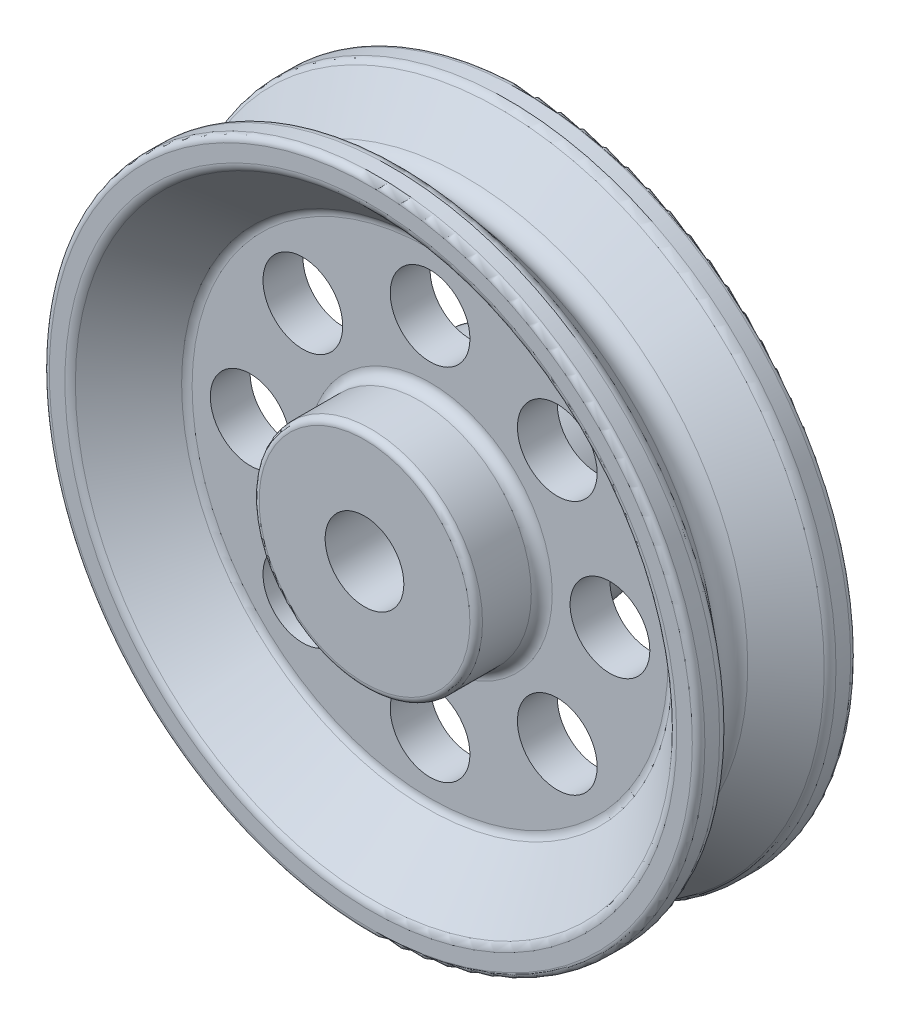
ISO-10303-21;
HEADER;
FILE_DESCRIPTION(('STEP AP214'),'2;1');
FILE_NAME('part.step','',(''),(''),'','','');
FILE_SCHEMA(('AUTOMOTIVE_DESIGN { 1 0 10303 214 1 1 1 1 }'));
ENDSEC;
DATA;
#1=APPLICATION_CONTEXT('core data for automotive mechanical design processes');
#2=APPLICATION_PROTOCOL_DEFINITION('international standard','automotive_design',2000,#1);
#3=PRODUCT_CONTEXT('',#1,'mechanical');
#4=PRODUCT('Part','Part','',(#3));
#5=PRODUCT_RELATED_PRODUCT_CATEGORY('part','',(#4));
#6=PRODUCT_DEFINITION_FORMATION('','',#4);
#7=PRODUCT_DEFINITION_CONTEXT('part definition',#1,'design');
#8=PRODUCT_DEFINITION('design','',#6,#7);
#9=PRODUCT_DEFINITION_SHAPE('','',#8);
#10=(LENGTH_UNIT() NAMED_UNIT(*) SI_UNIT(.MILLI.,.METRE.));
#11=(NAMED_UNIT(*) PLANE_ANGLE_UNIT() SI_UNIT($,.RADIAN.));
#12=(NAMED_UNIT(*) SI_UNIT($,.STERADIAN.) SOLID_ANGLE_UNIT());
#13=UNCERTAINTY_MEASURE_WITH_UNIT(LENGTH_MEASURE(1.E-05),#10,'distance_accuracy_value','');
#14=(GEOMETRIC_REPRESENTATION_CONTEXT(3) GLOBAL_UNCERTAINTY_ASSIGNED_CONTEXT((#13)) GLOBAL_UNIT_ASSIGNED_CONTEXT((#10,
#11,#12)) REPRESENTATION_CONTEXT('',''));
#15=CARTESIAN_POINT('',(0.,0.,0.));
#16=DIRECTION('',(0.,0.,1.));
#17=DIRECTION('',(1.,0.,0.));
#18=AXIS2_PLACEMENT_3D('',#15,#16,#17);
#19=CARTESIAN_POINT('',(0.,1.005,-0.815));
#20=DIRECTION('',(0.,0.,1.));
#21=DIRECTION('',(1.,0.,0.));
#22=AXIS2_PLACEMENT_3D('',#19,#20,#21);
#23=PLANE('',#22);
#24=CARTESIAN_POINT('',(0.,0.,-0.815));
#25=DIRECTION('',(0.,0.,1.));
#26=DIRECTION('',(1.,0.,0.));
#27=AXIS2_PLACEMENT_3D('',#24,#25,#26);
#28=CIRCLE('',#27,1.005);
#29=CARTESIAN_POINT('',(1.005,0.,-0.815));
#30=VERTEX_POINT('',#29);
#31=EDGE_CURVE('E79',#30,#30,#28,.T.);
#32=ORIENTED_EDGE('',*,*,#31,.F.);
#33=EDGE_LOOP('',(#32));
#34=FACE_BOUND('',#33,.T.);
#35=CARTESIAN_POINT('',(0.,0.,-0.815));
#36=DIRECTION('',(0.,0.,1.));
#37=DIRECTION('',(1.,0.,0.));
#38=AXIS2_PLACEMENT_3D('',#35,#36,#37);
#39=CIRCLE('',#38,0.375);
#40=CARTESIAN_POINT('',(0.375,0.,-0.815));
#41=VERTEX_POINT('',#40);
#42=EDGE_CURVE('E10',#41,#41,#39,.T.);
#43=ORIENTED_EDGE('',*,*,#42,.T.);
#44=EDGE_LOOP('',(#43));
#45=FACE_BOUND('',#44,.T.);
#46=ADVANCED_FACE('F40',(#34,#45),#23,.F.);
#47=CARTESIAN_POINT('',(0.,0.,29.1959860355186));
#48=DIRECTION('',(0.,0.,1.));
#49=DIRECTION('',(1.,0.,0.));
#50=AXIS2_PLACEMENT_3D('',#47,#48,#49);
#51=CYLINDRICAL_SURFACE('',#50,0.375);
#52=ORIENTED_EDGE('',*,*,#42,.F.);
#53=EDGE_LOOP('',(#52));
#54=FACE_BOUND('',#53,.T.);
#55=CARTESIAN_POINT('',(0.,0.,0.815));
#56=DIRECTION('',(0.,0.,1.));
#57=DIRECTION('',(1.,0.,0.));
#58=AXIS2_PLACEMENT_3D('',#55,#56,#57);
#59=CIRCLE('',#58,0.375);
#60=CARTESIAN_POINT('',(0.375,0.,0.815));
#61=VERTEX_POINT('',#60);
#62=EDGE_CURVE('E42',#61,#61,#59,.T.);
#63=ORIENTED_EDGE('',*,*,#62,.T.);
#64=EDGE_LOOP('',(#63));
#65=FACE_BOUND('',#64,.T.);
#66=ADVANCED_FACE('F318',(#54,#65),#51,.F.);
#67=CARTESIAN_POINT('',(0.,0.375,0.815));
#68=DIRECTION('',(0.,0.,-1.));
#69=DIRECTION('',(-1.,0.,0.));
#70=AXIS2_PLACEMENT_3D('',#67,#68,#69);
#71=PLANE('',#70);
#72=ORIENTED_EDGE('',*,*,#62,.F.);
#73=EDGE_LOOP('',(#72));
#74=FACE_BOUND('',#73,.T.);
#75=CARTESIAN_POINT('',(0.,0.,0.815));
#76=DIRECTION('',(0.,0.,1.));
#77=DIRECTION('',(1.,0.,0.));
#78=AXIS2_PLACEMENT_3D('',#75,#76,#77);
#79=CIRCLE('',#78,1.005);
#80=CARTESIAN_POINT('',(1.005,0.,0.815));
#81=VERTEX_POINT('',#80);
#82=EDGE_CURVE('E47',#81,#81,#79,.T.);
#83=ORIENTED_EDGE('',*,*,#82,.T.);
#84=EDGE_LOOP('',(#83));
#85=FACE_BOUND('',#84,.T.);
#86=ADVANCED_FACE('F159',(#74,#85),#71,.F.);
#87=CARTESIAN_POINT('',(0.,0.,0.755));
#88=DIRECTION('',(0.,0.,1.));
#89=DIRECTION('',(1.,0.,0.));
#90=AXIS2_PLACEMENT_3D('',#87,#88,#89);
#91=TOROIDAL_SURFACE('',#90,1.005,0.0599999999999999);
#92=ORIENTED_EDGE('',*,*,#82,.F.);
#93=EDGE_LOOP('',(#92));
#94=FACE_BOUND('',#93,.T.);
#95=CARTESIAN_POINT('',(0.,0.,0.754999999999999));
#96=DIRECTION('',(0.,0.,1.));
#97=DIRECTION('',(1.,0.,0.));
#98=AXIS2_PLACEMENT_3D('',#95,#96,#97);
#99=CIRCLE('',#98,1.065);
#100=CARTESIAN_POINT('',(1.065,0.,0.754999999999999));
#101=VERTEX_POINT('',#100);
#102=EDGE_CURVE('E154',#101,#101,#99,.T.);
#103=ORIENTED_EDGE('',*,*,#102,.T.);
#104=EDGE_LOOP('',(#103));
#105=FACE_BOUND('',#104,.T.);
#106=ADVANCED_FACE('F165',(#94,#105),#91,.T.);
#107=CARTESIAN_POINT('',(0.,0.,29.1959860355186));
#108=DIRECTION('',(0.,0.,1.));
#109=DIRECTION('',(1.,0.,0.));
#110=AXIS2_PLACEMENT_3D('',#107,#108,#109);
#111=CYLINDRICAL_SURFACE('',#110,1.065);
#112=ORIENTED_EDGE('',*,*,#102,.F.);
#113=EDGE_LOOP('',(#112));
#114=FACE_BOUND('',#113,.T.);
#115=CARTESIAN_POINT('',(0.,0.,0.290000000000002));
#116=DIRECTION('',(0.,0.,1.));
#117=DIRECTION('',(1.,0.,0.));
#118=AXIS2_PLACEMENT_3D('',#115,#116,#117);
#119=CIRCLE('',#118,1.065);
#120=CARTESIAN_POINT('',(1.065,0.,0.290000000000002));
#121=VERTEX_POINT('',#120);
#122=EDGE_CURVE('E155',#121,#121,#119,.T.);
#123=ORIENTED_EDGE('',*,*,#122,.T.);
#124=EDGE_LOOP('',(#123));
#125=FACE_BOUND('',#124,.T.);
#126=ADVANCED_FACE('F164',(#114,#125),#111,.T.);
#127=CARTESIAN_POINT('',(0.,0.,0.29));
#128=DIRECTION('',(0.,0.,1.));
#129=DIRECTION('',(1.,0.,0.));
#130=AXIS2_PLACEMENT_3D('',#127,#128,#129);
#131=TOROIDAL_SURFACE('',#130,1.165,0.1);
#132=ORIENTED_EDGE('',*,*,#122,.F.);
#133=EDGE_LOOP('',(#132));
#134=FACE_BOUND('',#133,.T.);
#135=CARTESIAN_POINT('',(0.,0.,0.189999999999999));
#136=DIRECTION('',(0.,0.,1.));
#137=DIRECTION('',(1.,0.,0.));
#138=AXIS2_PLACEMENT_3D('',#135,#136,#137);
#139=CIRCLE('',#138,1.165);
#140=CARTESIAN_POINT('',(1.165,0.,0.189999999999999));
#141=VERTEX_POINT('',#140);
#142=EDGE_CURVE('E149',#141,#141,#139,.T.);
#143=ORIENTED_EDGE('',*,*,#142,.T.);
#144=EDGE_LOOP('',(#143));
#145=FACE_BOUND('',#144,.T.);
#146=ADVANCED_FACE('F174',(#134,#145),#131,.F.);
#147=CARTESIAN_POINT('',(0.,1.165,0.19));
#148=DIRECTION('',(0.,0.,-1.));
#149=DIRECTION('',(-1.,0.,0.));
#150=AXIS2_PLACEMENT_3D('',#147,#148,#149);
#151=PLANE('',#150);
#152=CARTESIAN_POINT('',(1.21268812973493,1.21268812973493,0.19));
#153=DIRECTION('',(0.,0.,1.));
#154=DIRECTION('',(1.,0.,0.));
#155=AXIS2_PLACEMENT_3D('',#152,#153,#154);
#156=CIRCLE('',#155,0.38);
#157=CARTESIAN_POINT('',(1.59268812973493,1.21268812973493,0.19));
#158=VERTEX_POINT('',#157);
#159=EDGE_CURVE('E533',#158,#158,#156,.T.);
#160=ORIENTED_EDGE('',*,*,#159,.F.);
#161=EDGE_LOOP('',(#160));
#162=FACE_BOUND('',#161,.T.);
#163=CARTESIAN_POINT('',(1.715,0.,0.19));
#164=DIRECTION('',(0.,0.,1.));
#165=DIRECTION('',(1.,0.,0.));
#166=AXIS2_PLACEMENT_3D('',#163,#164,#165);
#167=CIRCLE('',#166,0.38);
#168=CARTESIAN_POINT('',(2.095,0.,0.19));
#169=VERTEX_POINT('',#168);
#170=EDGE_CURVE('E535',#169,#169,#167,.T.);
#171=ORIENTED_EDGE('',*,*,#170,.F.);
#172=EDGE_LOOP('',(#171));
#173=FACE_BOUND('',#172,.T.);
#174=CARTESIAN_POINT('',(1.21268812973493,-1.21268812973493,0.19));
#175=DIRECTION('',(0.,0.,1.));
#176=DIRECTION('',(1.,0.,0.));
#177=AXIS2_PLACEMENT_3D('',#174,#175,#176);
#178=CIRCLE('',#177,0.38);
#179=CARTESIAN_POINT('',(1.59268812973493,-1.21268812973493,0.19));
#180=VERTEX_POINT('',#179);
#181=EDGE_CURVE('E534',#180,#180,#178,.T.);
#182=ORIENTED_EDGE('',*,*,#181,.F.);
#183=EDGE_LOOP('',(#182));
#184=FACE_BOUND('',#183,.T.);
#185=CARTESIAN_POINT('',(0.,-1.715,0.19));
#186=DIRECTION('',(0.,0.,1.));
#187=DIRECTION('',(1.,0.,0.));
#188=AXIS2_PLACEMENT_3D('',#185,#186,#187);
#189=CIRCLE('',#188,0.38);
#190=CARTESIAN_POINT('',(0.38,-1.715,0.19));
#191=VERTEX_POINT('',#190);
#192=EDGE_CURVE('E537',#191,#191,#189,.T.);
#193=ORIENTED_EDGE('',*,*,#192,.F.);
#194=EDGE_LOOP('',(#193));
#195=FACE_BOUND('',#194,.T.);
#196=CARTESIAN_POINT('',(-1.21268812973493,-1.21268812973493,0.19));
#197=DIRECTION('',(0.,0.,1.));
#198=DIRECTION('',(1.,0.,0.));
#199=AXIS2_PLACEMENT_3D('',#196,#197,#198);
#200=CIRCLE('',#199,0.38);
#201=CARTESIAN_POINT('',(-0.832688129734929,-1.21268812973493,0.19));
#202=VERTEX_POINT('',#201);
#203=EDGE_CURVE('E545',#202,#202,#200,.T.);
#204=ORIENTED_EDGE('',*,*,#203,.F.);
#205=EDGE_LOOP('',(#204));
#206=FACE_BOUND('',#205,.T.);
#207=CARTESIAN_POINT('',(-1.715,0.,0.19));
#208=DIRECTION('',(0.,0.,1.));
#209=DIRECTION('',(1.,0.,0.));
#210=AXIS2_PLACEMENT_3D('',#207,#208,#209);
#211=CIRCLE('',#210,0.38);
#212=CARTESIAN_POINT('',(-1.335,0.,0.19));
#213=VERTEX_POINT('',#212);
#214=EDGE_CURVE('E544',#213,#213,#211,.T.);
#215=ORIENTED_EDGE('',*,*,#214,.F.);
#216=EDGE_LOOP('',(#215));
#217=FACE_BOUND('',#216,.T.);
#218=CARTESIAN_POINT('',(-1.21268812973493,1.21268812973493,0.19));
#219=DIRECTION('',(0.,0.,1.));
#220=DIRECTION('',(1.,0.,0.));
#221=AXIS2_PLACEMENT_3D('',#218,#219,#220);
#222=CIRCLE('',#221,0.38);
#223=CARTESIAN_POINT('',(-0.832688129734929,1.21268812973493,0.19));
#224=VERTEX_POINT('',#223);
#225=EDGE_CURVE('E547',#224,#224,#222,.T.);
#226=ORIENTED_EDGE('',*,*,#225,.F.);
#227=EDGE_LOOP('',(#226));
#228=FACE_BOUND('',#227,.T.);
#229=CARTESIAN_POINT('',(0.,1.715,0.19));
#230=DIRECTION('',(0.,0.,1.));
#231=DIRECTION('',(1.,0.,0.));
#232=AXIS2_PLACEMENT_3D('',#229,#230,#231);
#233=CIRCLE('',#232,0.38);
#234=CARTESIAN_POINT('',(0.38,1.715,0.19));
#235=VERTEX_POINT('',#234);
#236=EDGE_CURVE('E60',#235,#235,#233,.T.);
#237=ORIENTED_EDGE('',*,*,#236,.F.);
#238=EDGE_LOOP('',(#237));
#239=FACE_BOUND('',#238,.T.);
#240=ORIENTED_EDGE('',*,*,#142,.F.);
#241=EDGE_LOOP('',(#240));
#242=FACE_BOUND('',#241,.T.);
#243=CARTESIAN_POINT('',(0.,0.,0.189999999999999));
#244=DIRECTION('',(0.,0.,1.));
#245=DIRECTION('',(1.,0.,0.));
#246=AXIS2_PLACEMENT_3D('',#243,#244,#245);
#247=CIRCLE('',#246,2.26857864376269);
#248=CARTESIAN_POINT('',(2.26857864376269,0.,0.189999999999999));
#249=VERTEX_POINT('',#248);
#250=EDGE_CURVE('E148',#249,#249,#247,.T.);
#251=ORIENTED_EDGE('',*,*,#250,.T.);
#252=EDGE_LOOP('',(#251));
#253=FACE_BOUND('',#252,.T.);
#254=ADVANCED_FACE('F179',(#162,#173,#184,#195,#206,#217,#228,#239,#242,#253),#151,.F.);
#255=CARTESIAN_POINT('',(0.,0.,0.29));
#256=DIRECTION('',(0.,0.,1.));
#257=DIRECTION('',(1.,0.,0.));
#258=AXIS2_PLACEMENT_3D('',#255,#256,#257);
#259=TOROIDAL_SURFACE('',#258,2.26857864376269,0.0999999999999999);
#260=ORIENTED_EDGE('',*,*,#250,.F.);
#261=EDGE_LOOP('',(#260));
#262=FACE_BOUND('',#261,.T.);
#263=CARTESIAN_POINT('',(0.,0.,0.219289321881345));
#264=DIRECTION('',(0.,0.,1.));
#265=DIRECTION('',(1.,0.,0.));
#266=AXIS2_PLACEMENT_3D('',#263,#264,#265);
#267=CIRCLE('',#266,2.33928932188135);
#268=CARTESIAN_POINT('',(2.33928932188135,0.,0.219289321881345));
#269=VERTEX_POINT('',#268);
#270=EDGE_CURVE('E141',#269,#269,#267,.T.);
#271=ORIENTED_EDGE('',*,*,#270,.T.);
#272=EDGE_LOOP('',(#271));
#273=FACE_BOUND('',#272,.T.);
#274=ADVANCED_FACE('F181',(#262,#273),#259,.F.);
#275=CARTESIAN_POINT('',(0.,0.,0.725710678118652));
#276=DIRECTION('',(0.,0.,1.));
#277=DIRECTION('',(1.,0.,0.));
#278=AXIS2_PLACEMENT_3D('',#275,#276,#277);
#279=CONICAL_SURFACE('',#278,2.84571067811865,0.785398163397448);
#280=ORIENTED_EDGE('',*,*,#270,.F.);
#281=EDGE_LOOP('',(#280));
#282=FACE_BOUND('',#281,.T.);
#283=CARTESIAN_POINT('',(0.,0.,0.725710678118652));
#284=DIRECTION('',(0.,0.,1.));
#285=DIRECTION('',(1.,0.,0.));
#286=AXIS2_PLACEMENT_3D('',#283,#284,#285);
#287=CIRCLE('',#286,2.84571067811865);
#288=CARTESIAN_POINT('',(2.84571067811865,0.,0.725710678118652));
#289=VERTEX_POINT('',#288);
#290=EDGE_CURVE('E138',#289,#289,#287,.T.);
#291=ORIENTED_EDGE('',*,*,#290,.T.);
#292=EDGE_LOOP('',(#291));
#293=FACE_BOUND('',#292,.T.);
#294=ADVANCED_FACE('F187',(#282,#293),#279,.F.);
#295=CARTESIAN_POINT('',(0.,0.,0.655));
#296=DIRECTION('',(0.,0.,1.));
#297=DIRECTION('',(1.,0.,0.));
#298=AXIS2_PLACEMENT_3D('',#295,#296,#297);
#299=TOROIDAL_SURFACE('',#298,2.91642135623731,0.1);
#300=ORIENTED_EDGE('',*,*,#290,.F.);
#301=EDGE_LOOP('',(#300));
#302=FACE_BOUND('',#301,.T.);
#303=CARTESIAN_POINT('',(0.,0.,0.754999999999999));
#304=DIRECTION('',(0.,0.,1.));
#305=DIRECTION('',(1.,0.,0.));
#306=AXIS2_PLACEMENT_3D('',#303,#304,#305);
#307=CIRCLE('',#306,2.91642135623731);
#308=CARTESIAN_POINT('',(2.91642135623731,0.,0.754999999999999));
#309=VERTEX_POINT('',#308);
#310=EDGE_CURVE('E139',#309,#309,#307,.T.);
#311=ORIENTED_EDGE('',*,*,#310,.T.);
#312=EDGE_LOOP('',(#311));
#313=FACE_BOUND('',#312,.T.);
#314=ADVANCED_FACE('F198',(#302,#313),#299,.T.);
#315=CARTESIAN_POINT('',(0.,2.91642135623731,0.754999999999999));
#316=DIRECTION('',(0.,0.,-1.));
#317=DIRECTION('',(-1.,0.,0.));
#318=AXIS2_PLACEMENT_3D('',#315,#316,#317);
#319=PLANE('',#318);
#320=ORIENTED_EDGE('',*,*,#310,.F.);
#321=EDGE_LOOP('',(#320));
#322=FACE_BOUND('',#321,.T.);
#323=CARTESIAN_POINT('',(0.,0.,0.754999999999999));
#324=DIRECTION('',(0.,0.,1.));
#325=DIRECTION('',(1.,0.,0.));
#326=AXIS2_PLACEMENT_3D('',#323,#324,#325);
#327=CIRCLE('',#326,3.065);
#328=CARTESIAN_POINT('',(3.065,0.,0.754999999999999));
#329=VERTEX_POINT('',#328);
#330=EDGE_CURVE('E133',#329,#329,#327,.T.);
#331=ORIENTED_EDGE('',*,*,#330,.T.);
#332=EDGE_LOOP('',(#331));
#333=FACE_BOUND('',#332,.T.);
#334=ADVANCED_FACE('F205',(#322,#333),#319,.F.);
#335=CARTESIAN_POINT('',(0.,0.,0.694999999999999));
#336=DIRECTION('',(0.,0.,1.));
#337=DIRECTION('',(1.,0.,0.));
#338=AXIS2_PLACEMENT_3D('',#335,#336,#337);
#339=TOROIDAL_SURFACE('',#338,3.065,0.06);
#340=ORIENTED_EDGE('',*,*,#330,.F.);
#341=EDGE_LOOP('',(#340));
#342=FACE_BOUND('',#341,.T.);
#343=CARTESIAN_POINT('',(0.,0.,0.694999999999998));
#344=DIRECTION('',(0.,0.,1.));
#345=DIRECTION('',(1.,0.,0.));
#346=AXIS2_PLACEMENT_3D('',#343,#344,#345);
#347=CIRCLE('',#346,3.125);
#348=CARTESIAN_POINT('',(3.125,0.,0.694999999999998));
#349=VERTEX_POINT('',#348);
#350=EDGE_CURVE('E134',#349,#349,#347,.T.);
#351=ORIENTED_EDGE('',*,*,#350,.T.);
#352=EDGE_LOOP('',(#351));
#353=FACE_BOUND('',#352,.T.);
#354=ADVANCED_FACE('F208',(#342,#353),#339,.T.);
#355=CARTESIAN_POINT('',(0.,0.,29.1959860355186));
#356=DIRECTION('',(0.,0.,1.));
#357=DIRECTION('',(1.,0.,0.));
#358=AXIS2_PLACEMENT_3D('',#355,#356,#357);
#359=CYLINDRICAL_SURFACE('',#358,3.125);
#360=ORIENTED_EDGE('',*,*,#350,.F.);
#361=EDGE_LOOP('',(#360));
#362=FACE_BOUND('',#361,.T.);
#363=CARTESIAN_POINT('',(0.,0.,0.554779036453578));
#364=DIRECTION('',(0.,0.,1.));
#365=DIRECTION('',(1.,0.,0.));
#366=AXIS2_PLACEMENT_3D('',#363,#364,#365);
#367=CIRCLE('',#366,3.125);
#368=CARTESIAN_POINT('',(3.125,0.,0.554779036453578));
#369=VERTEX_POINT('',#368);
#370=EDGE_CURVE('E126',#369,#369,#367,.T.);
#371=ORIENTED_EDGE('',*,*,#370,.T.);
#372=EDGE_LOOP('',(#371));
#373=FACE_BOUND('',#372,.T.);
#374=ADVANCED_FACE('F212',(#362,#373),#359,.T.);
#375=CARTESIAN_POINT('',(0.,0.,0.554779036453579));
#376=DIRECTION('',(0.,0.,1.));
#377=DIRECTION('',(1.,0.,0.));
#378=AXIS2_PLACEMENT_3D('',#375,#376,#377);
#379=TOROIDAL_SURFACE('',#378,3.025,0.0999999999999998);
#380=ORIENTED_EDGE('',*,*,#370,.F.);
#381=EDGE_LOOP('',(#380));
#382=FACE_BOUND('',#381,.T.);
#383=CARTESIAN_POINT('',(0.,0.,0.478174592141681));
#384=DIRECTION('',(0.,0.,1.));
#385=DIRECTION('',(1.,0.,0.));
#386=AXIS2_PLACEMENT_3D('',#383,#384,#385);
#387=CIRCLE('',#386,3.08927876096865);
#388=CARTESIAN_POINT('',(3.08927876096865,0.,0.478174592141681));
#389=VERTEX_POINT('',#388);
#390=EDGE_CURVE('E123',#389,#389,#387,.T.);
#391=ORIENTED_EDGE('',*,*,#390,.T.);
#392=EDGE_LOOP('',(#391));
#393=FACE_BOUND('',#392,.T.);
#394=ADVANCED_FACE('F219',(#382,#393),#379,.T.);
#395=CARTESIAN_POINT('',(0.,0.,0.145548444192605));
#396=DIRECTION('',(0.,0.,1.));
#397=DIRECTION('',(1.,0.,0.));
#398=AXIS2_PLACEMENT_3D('',#395,#396,#397);
#399=CONICAL_SURFACE('',#398,2.69287035415956,0.872664625997176);
#400=ORIENTED_EDGE('',*,*,#390,.F.);
#401=EDGE_LOOP('',(#400));
#402=FACE_BOUND('',#401,.T.);
#403=CARTESIAN_POINT('',(0.,0.,0.145548444192605));
#404=DIRECTION('',(0.,0.,1.));
#405=DIRECTION('',(1.,0.,0.));
#406=AXIS2_PLACEMENT_3D('',#403,#404,#405);
#407=CIRCLE('',#406,2.69287035415956);
#408=CARTESIAN_POINT('',(2.69287035415956,0.,0.145548444192605));
#409=VERTEX_POINT('',#408);
#410=EDGE_CURVE('E124',#409,#409,#407,.T.);
#411=ORIENTED_EDGE('',*,*,#410,.T.);
#412=EDGE_LOOP('',(#411));
#413=FACE_BOUND('',#412,.T.);
#414=ADVANCED_FACE('F229',(#402,#413),#399,.T.);
#415=CARTESIAN_POINT('',(0.,0.,0.));
#416=DIRECTION('',(0.,0.,1.));
#417=DIRECTION('',(1.,0.,0.));
#418=AXIS2_PLACEMENT_3D('',#415,#416,#417);
#419=TOROIDAL_SURFACE('',#418,2.815,0.189999999999999);
#420=ORIENTED_EDGE('',*,*,#410,.F.);
#421=EDGE_LOOP('',(#420));
#422=FACE_BOUND('',#421,.T.);
#423=CARTESIAN_POINT('',(0.,0.,-0.145548444192605));
#424=DIRECTION('',(0.,0.,1.));
#425=DIRECTION('',(1.,0.,0.));
#426=AXIS2_PLACEMENT_3D('',#423,#424,#425);
#427=CIRCLE('',#426,2.69287035415956);
#428=CARTESIAN_POINT('',(2.69287035415956,0.,-0.145548444192605));
#429=VERTEX_POINT('',#428);
#430=EDGE_CURVE('E118',#429,#429,#427,.T.);
#431=ORIENTED_EDGE('',*,*,#430,.T.);
#432=EDGE_LOOP('',(#431));
#433=FACE_BOUND('',#432,.T.);
#434=ADVANCED_FACE('F234',(#422,#433),#419,.F.);
#435=CARTESIAN_POINT('',(0.,0.,-0.478174592141702));
#436=DIRECTION('',(0.,0.,-1.));
#437=DIRECTION('',(-1.,0.,0.));
#438=AXIS2_PLACEMENT_3D('',#435,#436,#437);
#439=CONICAL_SURFACE('',#438,3.08927876096866,0.872664625997154);
#440=ORIENTED_EDGE('',*,*,#430,.F.);
#441=EDGE_LOOP('',(#440));
#442=FACE_BOUND('',#441,.T.);
#443=CARTESIAN_POINT('',(0.,0.,-0.478174592141702));
#444=DIRECTION('',(0.,0.,1.));
#445=DIRECTION('',(1.,0.,0.));
#446=AXIS2_PLACEMENT_3D('',#443,#444,#445);
#447=CIRCLE('',#446,3.08927876096866);
#448=CARTESIAN_POINT('',(3.08927876096866,0.,-0.478174592141702));
#449=VERTEX_POINT('',#448);
#450=EDGE_CURVE('E119',#449,#449,#447,.T.);
#451=ORIENTED_EDGE('',*,*,#450,.T.);
#452=EDGE_LOOP('',(#451));
#453=FACE_BOUND('',#452,.T.);
#454=ADVANCED_FACE('F236',(#442,#453),#439,.T.);
#455=CARTESIAN_POINT('',(0.,0.,-0.554779036453598));
#456=DIRECTION('',(0.,0.,1.));
#457=DIRECTION('',(1.,0.,0.));
#458=AXIS2_PLACEMENT_3D('',#455,#456,#457);
#459=TOROIDAL_SURFACE('',#458,3.025,0.0999999999999998);
#460=ORIENTED_EDGE('',*,*,#450,.F.);
#461=EDGE_LOOP('',(#460));
#462=FACE_BOUND('',#461,.T.);
#463=CARTESIAN_POINT('',(0.,0.,-0.554779036453599));
#464=DIRECTION('',(0.,0.,1.));
#465=DIRECTION('',(1.,0.,0.));
#466=AXIS2_PLACEMENT_3D('',#463,#464,#465);
#467=CIRCLE('',#466,3.125);
#468=CARTESIAN_POINT('',(3.125,0.,-0.554779036453599));
#469=VERTEX_POINT('',#468);
#470=EDGE_CURVE('E114',#469,#469,#467,.T.);
#471=ORIENTED_EDGE('',*,*,#470,.T.);
#472=EDGE_LOOP('',(#471));
#473=FACE_BOUND('',#472,.T.);
#474=ADVANCED_FACE('F243',(#462,#473),#459,.T.);
#475=CARTESIAN_POINT('',(0.,0.,29.1959860355186));
#476=DIRECTION('',(0.,0.,1.));
#477=DIRECTION('',(1.,0.,0.));
#478=AXIS2_PLACEMENT_3D('',#475,#476,#477);
#479=CYLINDRICAL_SURFACE('',#478,3.125);
#480=ORIENTED_EDGE('',*,*,#470,.F.);
#481=EDGE_LOOP('',(#480));
#482=FACE_BOUND('',#481,.T.);
#483=CARTESIAN_POINT('',(0.,0.,-0.695000000000001));
#484=DIRECTION('',(0.,0.,1.));
#485=DIRECTION('',(1.,0.,0.));
#486=AXIS2_PLACEMENT_3D('',#483,#484,#485);
#487=CIRCLE('',#486,3.125);
#488=CARTESIAN_POINT('',(3.125,0.,-0.695000000000001));
#489=VERTEX_POINT('',#488);
#490=EDGE_CURVE('E109',#489,#489,#487,.T.);
#491=ORIENTED_EDGE('',*,*,#490,.T.);
#492=EDGE_LOOP('',(#491));
#493=FACE_BOUND('',#492,.T.);
#494=ADVANCED_FACE('F248',(#482,#493),#479,.T.);
#495=CARTESIAN_POINT('',(0.,0.,-0.695));
#496=DIRECTION('',(0.,0.,1.));
#497=DIRECTION('',(1.,0.,0.));
#498=AXIS2_PLACEMENT_3D('',#495,#496,#497);
#499=TOROIDAL_SURFACE('',#498,3.065,0.06);
#500=ORIENTED_EDGE('',*,*,#490,.F.);
#501=EDGE_LOOP('',(#500));
#502=FACE_BOUND('',#501,.T.);
#503=CARTESIAN_POINT('',(0.,0.,-0.754999999999999));
#504=DIRECTION('',(0.,0.,1.));
#505=DIRECTION('',(1.,0.,0.));
#506=AXIS2_PLACEMENT_3D('',#503,#504,#505);
#507=CIRCLE('',#506,3.065);
#508=CARTESIAN_POINT('',(3.065,0.,-0.754999999999999));
#509=VERTEX_POINT('',#508);
#510=EDGE_CURVE('E110',#509,#509,#507,.T.);
#511=ORIENTED_EDGE('',*,*,#510,.T.);
#512=EDGE_LOOP('',(#511));
#513=FACE_BOUND('',#512,.T.);
#514=ADVANCED_FACE('F258',(#502,#513),#499,.T.);
#515=CARTESIAN_POINT('',(0.,3.065,-0.755));
#516=DIRECTION('',(0.,0.,1.));
#517=DIRECTION('',(1.,0.,0.));
#518=AXIS2_PLACEMENT_3D('',#515,#516,#517);
#519=PLANE('',#518);
#520=ORIENTED_EDGE('',*,*,#510,.F.);
#521=EDGE_LOOP('',(#520));
#522=FACE_BOUND('',#521,.T.);
#523=CARTESIAN_POINT('',(0.,0.,-0.754999999999999));
#524=DIRECTION('',(0.,0.,1.));
#525=DIRECTION('',(1.,0.,0.));
#526=AXIS2_PLACEMENT_3D('',#523,#524,#525);
#527=CIRCLE('',#526,2.91642135623731);
#528=CARTESIAN_POINT('',(2.91642135623731,0.,-0.754999999999999));
#529=VERTEX_POINT('',#528);
#530=EDGE_CURVE('E102',#529,#529,#527,.T.);
#531=ORIENTED_EDGE('',*,*,#530,.T.);
#532=EDGE_LOOP('',(#531));
#533=FACE_BOUND('',#532,.T.);
#534=ADVANCED_FACE('F265',(#522,#533),#519,.F.);
#535=CARTESIAN_POINT('',(0.,0.,-0.655));
#536=DIRECTION('',(0.,0.,1.));
#537=DIRECTION('',(1.,0.,0.));
#538=AXIS2_PLACEMENT_3D('',#535,#536,#537);
#539=TOROIDAL_SURFACE('',#538,2.91642135623731,0.0999999999999999);
#540=ORIENTED_EDGE('',*,*,#530,.F.);
#541=EDGE_LOOP('',(#540));
#542=FACE_BOUND('',#541,.T.);
#543=CARTESIAN_POINT('',(0.,0.,-0.725710678118656));
#544=DIRECTION('',(0.,0.,1.));
#545=DIRECTION('',(1.,0.,0.));
#546=AXIS2_PLACEMENT_3D('',#543,#544,#545);
#547=CIRCLE('',#546,2.84571067811865);
#548=CARTESIAN_POINT('',(2.84571067811865,0.,-0.725710678118656));
#549=VERTEX_POINT('',#548);
#550=EDGE_CURVE('E101',#549,#549,#547,.T.);
#551=ORIENTED_EDGE('',*,*,#550,.T.);
#552=EDGE_LOOP('',(#551));
#553=FACE_BOUND('',#552,.T.);
#554=ADVANCED_FACE('F268',(#542,#553),#539,.T.);
#555=CARTESIAN_POINT('',(0.,0.,-0.219289321881345));
#556=DIRECTION('',(0.,0.,-1.));
#557=DIRECTION('',(-1.,0.,0.));
#558=AXIS2_PLACEMENT_3D('',#555,#556,#557);
#559=CONICAL_SURFACE('',#558,2.33928932188135,0.785398163397446);
#560=ORIENTED_EDGE('',*,*,#550,.F.);
#561=EDGE_LOOP('',(#560));
#562=FACE_BOUND('',#561,.T.);
#563=CARTESIAN_POINT('',(0.,0.,-0.219289321881345));
#564=DIRECTION('',(0.,0.,1.));
#565=DIRECTION('',(1.,0.,0.));
#566=AXIS2_PLACEMENT_3D('',#563,#564,#565);
#567=CIRCLE('',#566,2.33928932188135);
#568=CARTESIAN_POINT('',(2.33928932188135,0.,-0.219289321881345));
#569=VERTEX_POINT('',#568);
#570=EDGE_CURVE('E98',#569,#569,#567,.T.);
#571=ORIENTED_EDGE('',*,*,#570,.T.);
#572=EDGE_LOOP('',(#571));
#573=FACE_BOUND('',#572,.T.);
#574=ADVANCED_FACE('F273',(#562,#573),#559,.F.);
#575=CARTESIAN_POINT('',(0.,0.,-0.29));
#576=DIRECTION('',(0.,0.,1.));
#577=DIRECTION('',(1.,0.,0.));
#578=AXIS2_PLACEMENT_3D('',#575,#576,#577);
#579=TOROIDAL_SURFACE('',#578,2.26857864376269,0.0999999999999999);
#580=ORIENTED_EDGE('',*,*,#570,.F.);
#581=EDGE_LOOP('',(#580));
#582=FACE_BOUND('',#581,.T.);
#583=CARTESIAN_POINT('',(0.,0.,-0.189999999999999));
#584=DIRECTION('',(0.,0.,1.));
#585=DIRECTION('',(1.,0.,0.));
#586=AXIS2_PLACEMENT_3D('',#583,#584,#585);
#587=CIRCLE('',#586,2.26857864376269);
#588=CARTESIAN_POINT('',(2.26857864376269,0.,-0.189999999999999));
#589=VERTEX_POINT('',#588);
#590=EDGE_CURVE('E92',#589,#589,#587,.T.);
#591=ORIENTED_EDGE('',*,*,#590,.T.);
#592=EDGE_LOOP('',(#591));
#593=FACE_BOUND('',#592,.T.);
#594=ADVANCED_FACE('F278',(#582,#593),#579,.F.);
#595=CARTESIAN_POINT('',(0.,2.26857864376269,-0.19));
#596=DIRECTION('',(0.,0.,1.));
#597=DIRECTION('',(1.,0.,0.));
#598=AXIS2_PLACEMENT_3D('',#595,#596,#597);
#599=PLANE('',#598);
#600=CARTESIAN_POINT('',(1.21268812973493,1.21268812973493,-0.19));
#601=DIRECTION('',(0.,0.,1.));
#602=DIRECTION('',(1.,0.,0.));
#603=AXIS2_PLACEMENT_3D('',#600,#601,#602);
#604=CIRCLE('',#603,0.38);
#605=CARTESIAN_POINT('',(1.59268812973493,1.21268812973493,-0.19));
#606=VERTEX_POINT('',#605);
#607=EDGE_CURVE('E37',#606,#606,#604,.T.);
#608=ORIENTED_EDGE('',*,*,#607,.T.);
#609=EDGE_LOOP('',(#608));
#610=FACE_BOUND('',#609,.T.);
#611=CARTESIAN_POINT('',(1.715,0.,-0.19));
#612=DIRECTION('',(0.,0.,1.));
#613=DIRECTION('',(1.,0.,0.));
#614=AXIS2_PLACEMENT_3D('',#611,#612,#613);
#615=CIRCLE('',#614,0.38);
#616=CARTESIAN_POINT('',(2.095,0.,-0.19));
#617=VERTEX_POINT('',#616);
#618=EDGE_CURVE('E72',#617,#617,#615,.T.);
#619=ORIENTED_EDGE('',*,*,#618,.T.);
#620=EDGE_LOOP('',(#619));
#621=FACE_BOUND('',#620,.T.);
#622=CARTESIAN_POINT('',(1.21268812973493,-1.21268812973493,-0.19));
#623=DIRECTION('',(0.,0.,1.));
#624=DIRECTION('',(1.,0.,0.));
#625=AXIS2_PLACEMENT_3D('',#622,#623,#624);
#626=CIRCLE('',#625,0.38);
#627=CARTESIAN_POINT('',(1.59268812973493,-1.21268812973493,-0.19));
#628=VERTEX_POINT('',#627);
#629=EDGE_CURVE('E66',#628,#628,#626,.T.);
#630=ORIENTED_EDGE('',*,*,#629,.T.);
#631=EDGE_LOOP('',(#630));
#632=FACE_BOUND('',#631,.T.);
#633=CARTESIAN_POINT('',(0.,-1.715,-0.19));
#634=DIRECTION('',(0.,0.,1.));
#635=DIRECTION('',(1.,0.,0.));
#636=AXIS2_PLACEMENT_3D('',#633,#634,#635);
#637=CIRCLE('',#636,0.38);
#638=CARTESIAN_POINT('',(0.38,-1.715,-0.19));
#639=VERTEX_POINT('',#638);
#640=EDGE_CURVE('E67',#639,#639,#637,.T.);
#641=ORIENTED_EDGE('',*,*,#640,.T.);
#642=EDGE_LOOP('',(#641));
#643=FACE_BOUND('',#642,.T.);
#644=CARTESIAN_POINT('',(-1.21268812973493,-1.21268812973493,-0.19));
#645=DIRECTION('',(0.,0.,1.));
#646=DIRECTION('',(1.,0.,0.));
#647=AXIS2_PLACEMENT_3D('',#644,#645,#646);
#648=CIRCLE('',#647,0.38);
#649=CARTESIAN_POINT('',(-0.832688129734929,-1.21268812973493,-0.19));
#650=VERTEX_POINT('',#649);
#651=EDGE_CURVE('E65',#650,#650,#648,.T.);
#652=ORIENTED_EDGE('',*,*,#651,.T.);
#653=EDGE_LOOP('',(#652));
#654=FACE_BOUND('',#653,.T.);
#655=CARTESIAN_POINT('',(-1.715,0.,-0.19));
#656=DIRECTION('',(0.,0.,1.));
#657=DIRECTION('',(1.,0.,0.));
#658=AXIS2_PLACEMENT_3D('',#655,#656,#657);
#659=CIRCLE('',#658,0.38);
#660=CARTESIAN_POINT('',(-1.335,0.,-0.19));
#661=VERTEX_POINT('',#660);
#662=EDGE_CURVE('E58',#661,#661,#659,.T.);
#663=ORIENTED_EDGE('',*,*,#662,.T.);
#664=EDGE_LOOP('',(#663));
#665=FACE_BOUND('',#664,.T.);
#666=CARTESIAN_POINT('',(-1.21268812973493,1.21268812973493,-0.19));
#667=DIRECTION('',(0.,0.,1.));
#668=DIRECTION('',(1.,0.,0.));
#669=AXIS2_PLACEMENT_3D('',#666,#667,#668);
#670=CIRCLE('',#669,0.38);
#671=CARTESIAN_POINT('',(-0.832688129734929,1.21268812973493,-0.19));
#672=VERTEX_POINT('',#671);
#673=EDGE_CURVE('E57',#672,#672,#670,.T.);
#674=ORIENTED_EDGE('',*,*,#673,.T.);
#675=EDGE_LOOP('',(#674));
#676=FACE_BOUND('',#675,.T.);
#677=CARTESIAN_POINT('',(0.,1.715,-0.19));
#678=DIRECTION('',(0.,0.,1.));
#679=DIRECTION('',(1.,0.,0.));
#680=AXIS2_PLACEMENT_3D('',#677,#678,#679);
#681=CIRCLE('',#680,0.38);
#682=CARTESIAN_POINT('',(0.38,1.715,-0.19));
#683=VERTEX_POINT('',#682);
#684=EDGE_CURVE('E52',#683,#683,#681,.T.);
#685=ORIENTED_EDGE('',*,*,#684,.T.);
#686=EDGE_LOOP('',(#685));
#687=FACE_BOUND('',#686,.T.);
#688=ORIENTED_EDGE('',*,*,#590,.F.);
#689=EDGE_LOOP('',(#688));
#690=FACE_BOUND('',#689,.T.);
#691=CARTESIAN_POINT('',(0.,0.,-0.189999999999999));
#692=DIRECTION('',(0.,0.,1.));
#693=DIRECTION('',(1.,0.,0.));
#694=AXIS2_PLACEMENT_3D('',#691,#692,#693);
#695=CIRCLE('',#694,1.165);
#696=CARTESIAN_POINT('',(1.165,0.,-0.189999999999999));
#697=VERTEX_POINT('',#696);
#698=EDGE_CURVE('E95',#697,#697,#695,.T.);
#699=ORIENTED_EDGE('',*,*,#698,.T.);
#700=EDGE_LOOP('',(#699));
#701=FACE_BOUND('',#700,.T.);
#702=ADVANCED_FACE('F287',(#610,#621,#632,#643,#654,#665,#676,#687,#690,#701),#599,.F.);
#703=CARTESIAN_POINT('',(0.,0.,-0.29));
#704=DIRECTION('',(0.,0.,1.));
#705=DIRECTION('',(1.,0.,0.));
#706=AXIS2_PLACEMENT_3D('',#703,#704,#705);
#707=TOROIDAL_SURFACE('',#706,1.165,0.1);
#708=ORIENTED_EDGE('',*,*,#698,.F.);
#709=EDGE_LOOP('',(#708));
#710=FACE_BOUND('',#709,.T.);
#711=CARTESIAN_POINT('',(0.,0.,-0.290000000000002));
#712=DIRECTION('',(0.,0.,1.));
#713=DIRECTION('',(1.,0.,0.));
#714=AXIS2_PLACEMENT_3D('',#711,#712,#713);
#715=CIRCLE('',#714,1.065);
#716=CARTESIAN_POINT('',(1.065,0.,-0.290000000000002));
#717=VERTEX_POINT('',#716);
#718=EDGE_CURVE('E83',#717,#717,#715,.T.);
#719=ORIENTED_EDGE('',*,*,#718,.T.);
#720=EDGE_LOOP('',(#719));
#721=FACE_BOUND('',#720,.T.);
#722=ADVANCED_FACE('F295',(#710,#721),#707,.F.);
#723=CARTESIAN_POINT('',(0.,0.,29.1959860355186));
#724=DIRECTION('',(0.,0.,1.));
#725=DIRECTION('',(1.,0.,0.));
#726=AXIS2_PLACEMENT_3D('',#723,#724,#725);
#727=CYLINDRICAL_SURFACE('',#726,1.065);
#728=ORIENTED_EDGE('',*,*,#718,.F.);
#729=EDGE_LOOP('',(#728));
#730=FACE_BOUND('',#729,.T.);
#731=CARTESIAN_POINT('',(0.,0.,-0.754999999999999));
#732=DIRECTION('',(0.,0.,1.));
#733=DIRECTION('',(1.,0.,0.));
#734=AXIS2_PLACEMENT_3D('',#731,#732,#733);
#735=CIRCLE('',#734,1.065);
#736=CARTESIAN_POINT('',(1.065,0.,-0.754999999999999));
#737=VERTEX_POINT('',#736);
#738=EDGE_CURVE('E77',#737,#737,#735,.T.);
#739=ORIENTED_EDGE('',*,*,#738,.T.);
#740=EDGE_LOOP('',(#739));
#741=FACE_BOUND('',#740,.T.);
#742=ADVANCED_FACE('F300',(#730,#741),#727,.T.);
#743=CARTESIAN_POINT('',(0.,0.,-0.755));
#744=DIRECTION('',(0.,0.,1.));
#745=DIRECTION('',(1.,0.,0.));
#746=AXIS2_PLACEMENT_3D('',#743,#744,#745);
#747=TOROIDAL_SURFACE('',#746,1.005,0.0599999999999999);
#748=ORIENTED_EDGE('',*,*,#738,.F.);
#749=EDGE_LOOP('',(#748));
#750=FACE_BOUND('',#749,.T.);
#751=ORIENTED_EDGE('',*,*,#31,.T.);
#752=EDGE_LOOP('',(#751));
#753=FACE_BOUND('',#752,.T.);
#754=ADVANCED_FACE('F301',(#750,#753),#747,.T.);
#755=CARTESIAN_POINT('',(0.,1.715,-0.815));
#756=DIRECTION('',(0.,0.,1.));
#757=DIRECTION('',(1.,0.,0.));
#758=AXIS2_PLACEMENT_3D('',#755,#756,#757);
#759=CYLINDRICAL_SURFACE('',#758,0.38);
#760=ORIENTED_EDGE('',*,*,#236,.T.);
#761=EDGE_LOOP('',(#760));
#762=FACE_BOUND('',#761,.T.);
#763=ORIENTED_EDGE('',*,*,#684,.F.);
#764=EDGE_LOOP('',(#763));
#765=FACE_BOUND('',#764,.T.);
#766=ADVANCED_FACE('F310',(#762,#765),#759,.F.);
#767=CARTESIAN_POINT('',(-1.21268812973493,1.21268812973493,-0.815));
#768=DIRECTION('',(0.,0.,1.));
#769=DIRECTION('',(1.,0.,0.));
#770=AXIS2_PLACEMENT_3D('',#767,#768,#769);
#771=CYLINDRICAL_SURFACE('',#770,0.38);
#772=ORIENTED_EDGE('',*,*,#225,.T.);
#773=EDGE_LOOP('',(#772));
#774=FACE_BOUND('',#773,.T.);
#775=ORIENTED_EDGE('',*,*,#673,.F.);
#776=EDGE_LOOP('',(#775));
#777=FACE_BOUND('',#776,.T.);
#778=ADVANCED_FACE('F314',(#774,#777),#771,.F.);
#779=CARTESIAN_POINT('',(-1.715,0.,-0.815));
#780=DIRECTION('',(0.,0.,1.));
#781=DIRECTION('',(1.,0.,0.));
#782=AXIS2_PLACEMENT_3D('',#779,#780,#781);
#783=CYLINDRICAL_SURFACE('',#782,0.38);
#784=ORIENTED_EDGE('',*,*,#214,.T.);
#785=EDGE_LOOP('',(#784));
#786=FACE_BOUND('',#785,.T.);
#787=ORIENTED_EDGE('',*,*,#662,.F.);
#788=EDGE_LOOP('',(#787));
#789=FACE_BOUND('',#788,.T.);
#790=ADVANCED_FACE('F462',(#786,#789),#783,.F.);
#791=CARTESIAN_POINT('',(-1.21268812973493,-1.21268812973493,-0.815));
#792=DIRECTION('',(0.,0.,1.));
#793=DIRECTION('',(1.,0.,0.));
#794=AXIS2_PLACEMENT_3D('',#791,#792,#793);
#795=CYLINDRICAL_SURFACE('',#794,0.38);
#796=ORIENTED_EDGE('',*,*,#203,.T.);
#797=EDGE_LOOP('',(#796));
#798=FACE_BOUND('',#797,.T.);
#799=ORIENTED_EDGE('',*,*,#651,.F.);
#800=EDGE_LOOP('',(#799));
#801=FACE_BOUND('',#800,.T.);
#802=ADVANCED_FACE('F474',(#798,#801),#795,.F.);
#803=CARTESIAN_POINT('',(0.,-1.715,-0.815));
#804=DIRECTION('',(0.,0.,1.));
#805=DIRECTION('',(1.,0.,0.));
#806=AXIS2_PLACEMENT_3D('',#803,#804,#805);
#807=CYLINDRICAL_SURFACE('',#806,0.38);
#808=ORIENTED_EDGE('',*,*,#192,.T.);
#809=EDGE_LOOP('',(#808));
#810=FACE_BOUND('',#809,.T.);
#811=ORIENTED_EDGE('',*,*,#640,.F.);
#812=EDGE_LOOP('',(#811));
#813=FACE_BOUND('',#812,.T.);
#814=ADVANCED_FACE('F484',(#810,#813),#807,.F.);
#815=CARTESIAN_POINT('',(1.21268812973493,-1.21268812973493,-0.815));
#816=DIRECTION('',(0.,0.,1.));
#817=DIRECTION('',(1.,0.,0.));
#818=AXIS2_PLACEMENT_3D('',#815,#816,#817);
#819=CYLINDRICAL_SURFACE('',#818,0.38);
#820=ORIENTED_EDGE('',*,*,#181,.T.);
#821=EDGE_LOOP('',(#820));
#822=FACE_BOUND('',#821,.T.);
#823=ORIENTED_EDGE('',*,*,#629,.F.);
#824=EDGE_LOOP('',(#823));
#825=FACE_BOUND('',#824,.T.);
#826=ADVANCED_FACE('F494',(#822,#825),#819,.F.);
#827=CARTESIAN_POINT('',(1.715,0.,-0.815));
#828=DIRECTION('',(0.,0.,1.));
#829=DIRECTION('',(1.,0.,0.));
#830=AXIS2_PLACEMENT_3D('',#827,#828,#829);
#831=CYLINDRICAL_SURFACE('',#830,0.38);
#832=ORIENTED_EDGE('',*,*,#170,.T.);
#833=EDGE_LOOP('',(#832));
#834=FACE_BOUND('',#833,.T.);
#835=ORIENTED_EDGE('',*,*,#618,.F.);
#836=EDGE_LOOP('',(#835));
#837=FACE_BOUND('',#836,.T.);
#838=ADVANCED_FACE('F502',(#834,#837),#831,.F.);
#839=CARTESIAN_POINT('',(1.21268812973493,1.21268812973493,-0.815));
#840=DIRECTION('',(0.,0.,1.));
#841=DIRECTION('',(1.,0.,0.));
#842=AXIS2_PLACEMENT_3D('',#839,#840,#841);
#843=CYLINDRICAL_SURFACE('',#842,0.38);
#844=ORIENTED_EDGE('',*,*,#159,.T.);
#845=EDGE_LOOP('',(#844));
#846=FACE_BOUND('',#845,.T.);
#847=ORIENTED_EDGE('',*,*,#607,.F.);
#848=EDGE_LOOP('',(#847));
#849=FACE_BOUND('',#848,.T.);
#850=ADVANCED_FACE('F513',(#846,#849),#843,.F.);
#851=CLOSED_SHELL('',(#46,#66,#86,#106,#126,#146,#254,#274,#294,#314,#334,#354,#374,#394,#414,
#434,#454,#474,#494,#514,#534,#554,#574,#594,#702,#722,#742,#754,#766,#778,#790,#802,#814,#826,
#838,#850));
#852=MANIFOLD_SOLID_BREP('B2',#851);
#853=ADVANCED_BREP_SHAPE_REPRESENTATION('',(#18,#852),#14);
#854=SHAPE_DEFINITION_REPRESENTATION(#9,#853);
ENDSEC;
END-ISO-10303-21;
